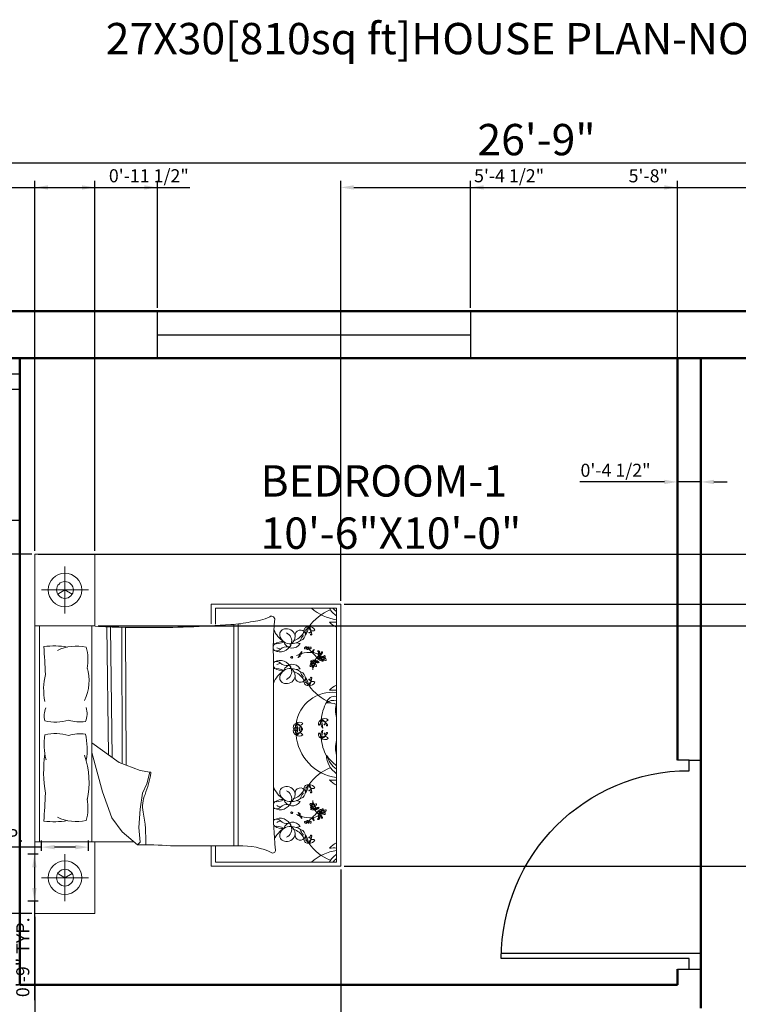
# Model space of a CAD drawing. Units: inches. Extents: x 3242 to 3618, y 1365 to 1814.
# Tile 5 of 6: x 3333 to 3471, y 1626 to 1814. Entities that reach past the tile are written whole.
import ezdxf

# ---------------------------------------------------------------- set-up
doc = ezdxf.new("R2010")
doc.units = ezdxf.units.IN
for name, color, linetype, lineweight in [('A-ANNO-DIMS', 2, 'Continuous', 18), ('A-ANNO-TEXT', 7, 'Continuous', 25), ('A-AREA-IDEN', 7, 'Continuous', 25), ('A-DOOR', 4, 'Continuous', 25), ('A-FURN', 8, 'Continuous', 18), ('A-GLAZ', 5, 'Continuous', 25), ('A-WALL', 7, 'Continuous', 50)]:
    doc.layers.add(name, color=color, linetype=linetype, lineweight=lineweight)
doc.styles.get("Standard").update_dxf_attribs({"font": 'arial.ttf'})
doc.dimstyles.new('ISO-25', dxfattribs={"dimtxt": 2.5, "dimasz": 2.5, "dimexe": 1.25, "dimexo": 0.625, "dimtad": 1, "dimdec": 0, "dimlunit": 3, "dimtxsty": 'Standard', "dimcen": 2.5, "dimadec": 0, "dimazin": 0, "dimtfac": 1, "dimtdec": 0, "dimtmove": 0, "dimatfit": 3, "dimfxl": 1, "dimarcsym": 0})

# ---------------------------------------------------------------- blocks, each defined once
blk = doc.blocks.new('*D3')
at = {"layer": 'A-ANNO-DIMS', "color": 0, "lineweight": -2, "transparency": 16777216}
for p, q in [((3271.48, 1759.28), (3271.48, 1788.3)), ((3592.48, 1759.28), (3592.48, 1788.3)), ((3273.98, 1787.05), (3589.98, 1787.05))]:
    blk.add_line(p, q, dxfattribs=at)
at = {"layer": 'A-ANNO-DIMS', "color": 0, "transparency": 16777216}
for points in [[(3273.98, 1787.47), (3273.98, 1786.64), (3271.48, 1787.05)], [(3589.98, 1787.47), (3589.98, 1786.64), (3592.48, 1787.05)]]:
    blk.add_solid(points, dxfattribs=at)
at = {"layer": 'Defpoints', "color": 0, "transparency": 16777216}
for p in [(3592.48, 1787.05), (3271.48, 1758.66), (3592.48, 1758.66)]:
    blk.add_point(p, dxfattribs=at)
at = {"layer": 'A-ANNO-DIMS', "color": 0, "transparency": 16777216, "insert": (3431.98, 1790.74), "char_height": 6, "attachment_point": 5}
blk.add_mtext('26\'-9"', dxfattribs=at)
blk = doc.blocks.new('DOOR-SWING-24IN')
for p, q in [((21.75, 28), (26.25, 28)), ((24, 28), (24, 26)), ((24, 26), (0, 26)), ((26.25, 25), (0, 25)), ((24, 2), (24, 0)), ((24, 0), (21.75, 0)), ((24, 0), (26.25, 0))]:
    blk.add_line(p, q)
blk.add_arc((24, 26), 24, 180, 270)
blk = doc.blocks.new('DOOR-SWING-36IN')
for p, q in [((33.75, 40), (38.25, 40)), ((36, 40), (36, 38)), ((36, 38), (0, 38)), ((38.25, 37), (0, 37)), ((36, 2), (36, 0)), ((36, 0), (33.75, 0)), ((36, 0), (38.25, 0))]:
    blk.add_line(p, q)
blk.add_arc((36, 38), 36, 180, 270)
blk = doc.blocks.new('WINDOW-60IN')
for p, q in [((0, 9), (60, 9)), ((0, 0), (0, 9)), ((60, 9), (60, 0)), ((0, 4.5), (60, 4.5)), ((60, 0), (0, 0))]:
    blk.add_line(p, q)
blk = doc.blocks.new('BEDSIDE-LAMP-SM')
for p, q in [((4.5, 0), (4.5, 9)), ((9, 4.5), (0, 4.5))]:
    blk.add_line(p, q)
for points in [[(4.5, 4.5), (3.11, 3.7)], [(4.5, 4.5), (5.89, 3.7)]]:
    blk.add_lwpolyline(points)
for radius in [3.21, 1.61]:
    blk.add_circle((4.5, 4.5), radius)
blk = doc.blocks.new('*D29')
at = {"layer": 'A-ANNO-DIMS', "color": 0, "lineweight": -2, "transparency": 16777216}
for p, q in [((3337.15, 1656.02), (3307.79, 1656.02)), ((3337.15, 1655.29), (3337.15, 1657.27)), ((3343.65, 1656.02), (3339.65, 1656.02)), ((3346.15, 1655.29), (3346.15, 1657.27))]:
    blk.add_line(p, q, dxfattribs=at)
at = {"layer": 'A-ANNO-DIMS', "color": 0, "transparency": 16777216}
for points in [[(3339.65, 1656.43), (3339.65, 1655.6), (3337.15, 1656.02)], [(3343.65, 1656.43), (3343.65, 1655.6), (3346.15, 1656.02)]]:
    blk.add_solid(points, dxfattribs=at)
at = {"layer": 'Defpoints', "color": 0, "transparency": 16777216}
for p in [(3337.15, 1656.02), (3337.15, 1654.67), (3346.15, 1654.67)]:
    blk.add_point(p, dxfattribs=at)
at = {"layer": 'A-ANNO-DIMS', "color": 0, "transparency": 16777216, "insert": (3321.22, 1657.92), "char_height": 2.5, "attachment_point": 5}
blk.add_mtext('LAMP 0\'-9" TYP.', dxfattribs=at)
blk = doc.blocks.new('*D30')
at = {"layer": 'A-ANNO-DIMS', "color": 0, "lineweight": -2, "transparency": 16777216}
for p, q in [((3336.53, 1654.67), (3334.55, 1654.67)), ((3335.8, 1652.17), (3335.8, 1648.17)), ((3336.53, 1645.67), (3334.55, 1645.67)), ((3335.8, 1645.67), (3335.8, 1626.68))]:
    blk.add_line(p, q, dxfattribs=at)
at = {"layer": 'A-ANNO-DIMS', "color": 0, "transparency": 16777216}
for points in [[(3335.39, 1652.17), (3336.22, 1652.17), (3335.8, 1654.67)], [(3335.39, 1648.17), (3336.22, 1648.17), (3335.8, 1645.67)]]:
    blk.add_solid(points, dxfattribs=at)
at = {"layer": 'Defpoints', "color": 0, "transparency": 16777216}
for p in [(3337.15, 1654.67), (3335.8, 1645.67), (3337.15, 1645.67)]:
    blk.add_point(p, dxfattribs=at)
at = {"layer": 'A-ANNO-DIMS', "color": 0, "transparency": 16777216, "insert": (3333.9, 1634.92), "char_height": 2.5, "attachment_point": 5, "rotation": 90}
blk.add_mtext('0\'-9" TYP.', dxfattribs=at)
blk = doc.blocks.new('*D33')
at = {"layer": 'A-ANNO-DIMS', "color": 0, "lineweight": -2, "transparency": 16777216}
for p, q in [((3271.48, 1759.28), (3271.48, 1783.61)), ((3273.98, 1782.36), (3356.86, 1782.36)), ((3359.36, 1759.28), (3359.36, 1783.61))]:
    blk.add_line(p, q, dxfattribs=at)
at = {"layer": 'A-ANNO-DIMS', "color": 0, "transparency": 16777216}
for points in [[(3273.98, 1782.77), (3273.98, 1781.94), (3271.48, 1782.36)], [(3356.86, 1782.77), (3356.86, 1781.94), (3359.36, 1782.36)]]:
    blk.add_solid(points, dxfattribs=at)
at = {"layer": 'Defpoints', "color": 0, "transparency": 16777216}
for p in [(3359.36, 1782.36), (3271.48, 1758.66), (3359.36, 1758.66)]:
    blk.add_point(p, dxfattribs=at)
at = {"layer": 'A-ANNO-DIMS', "color": 0, "transparency": 16777216, "insert": (3315.42, 1784.23), "char_height": 2.5, "attachment_point": 5}
blk.add_mtext('7\'-4"', dxfattribs=at)
blk = doc.blocks.new('*D34')
at = {"layer": 'A-ANNO-DIMS', "color": 0, "lineweight": -2, "transparency": 16777216}
for p, q in [((3419.36, 1759.28), (3419.36, 1783.61)), ((3421.86, 1782.36), (3484.93, 1782.36)), ((3487.43, 1759.28), (3487.43, 1783.61))]:
    blk.add_line(p, q, dxfattribs=at)
at = {"layer": 'A-ANNO-DIMS', "color": 0, "transparency": 16777216}
for points in [[(3421.86, 1782.77), (3421.86, 1781.94), (3419.36, 1782.36)], [(3484.93, 1782.77), (3484.93, 1781.94), (3487.43, 1782.36)]]:
    blk.add_solid(points, dxfattribs=at)
at = {"layer": 'Defpoints', "color": 0, "transparency": 16777216}
for p in [(3487.43, 1782.36), (3419.36, 1758.66), (3487.43, 1758.66)]:
    blk.add_point(p, dxfattribs=at)
at = {"layer": 'A-ANNO-DIMS', "color": 0, "transparency": 16777216, "insert": (3453.39, 1784.26), "char_height": 2.5, "attachment_point": 5}
blk.add_mtext('5\'-8"', dxfattribs=at)
blk = doc.blocks.new('*D47')
at = {"layer": 'A-ANNO-DIMS', "color": 0, "lineweight": -2, "transparency": 16777216}
for p, q in [((3458.98, 1749.03), (3458.98, 1724.71)), ((3463.48, 1749.03), (3463.48, 1724.71)), ((3456.48, 1725.96), (3440.26, 1725.96)), ((3463.48, 1725.96), (3458.98, 1725.96)), ((3465.98, 1725.96), (3468.48, 1725.96))]:
    blk.add_line(p, q, dxfattribs=at)
at = {"layer": 'A-ANNO-DIMS', "color": 0, "transparency": 16777216}
for points in [[(3456.48, 1726.37), (3456.48, 1725.54), (3458.98, 1725.96)], [(3465.98, 1726.37), (3465.98, 1725.54), (3463.48, 1725.96)]]:
    blk.add_solid(points, dxfattribs=at)
at = {"layer": 'Defpoints', "color": 0, "transparency": 16777216}
for p in [(3458.98, 1749.66), (3463.48, 1749.66), (3458.98, 1725.96)]:
    blk.add_point(p, dxfattribs=at)
at = {"layer": 'A-ANNO-DIMS', "color": 0, "transparency": 16777216, "insert": (3447.12, 1727.87), "char_height": 2.5, "attachment_point": 5}
blk.add_mtext('0\'-4 1/2"', dxfattribs=at)
blk = doc.blocks.new('*D48')
at = {"layer": 'A-ANNO-DIMS', "color": 0, "lineweight": -2, "transparency": 16777216}
for p, q in [((3394.48, 1651.75), (3394.48, 1376.71)), ((3335.91, 1642.66), (3335.91, 1376.71)), ((3338.41, 1377.96), (3391.98, 1377.96))]:
    blk.add_line(p, q, dxfattribs=at)
at = {"layer": 'A-ANNO-DIMS', "color": 0, "transparency": 16777216}
for points in [[(3338.41, 1378.37), (3338.41, 1377.54), (3335.91, 1377.96)], [(3391.98, 1378.37), (3391.98, 1377.54), (3394.48, 1377.96)]]:
    blk.add_solid(points, dxfattribs=at)
at = {"layer": 'Defpoints', "color": 0, "transparency": 16777216}
for p in [(3394.48, 1652.37), (3335.91, 1643.28), (3394.48, 1377.96)]:
    blk.add_point(p, dxfattribs=at)
at = {"layer": 'A-ANNO-DIMS', "color": 0, "transparency": 16777216, "insert": (3365.2, 1379.87), "char_height": 2.5, "attachment_point": 5}
blk.add_mtext('4\'-10 1/2"', dxfattribs=at)
blk = doc.blocks.new('*D49')
at = {"layer": 'A-ANNO-DIMS', "color": 0, "lineweight": -2, "transparency": 16777216}
for p, q in [((3395.11, 1702.58), (3617.43, 1702.58)), ((3616.18, 1700.08), (3616.18, 1654.87)), ((3395.11, 1652.37), (3617.43, 1652.37))]:
    blk.add_line(p, q, dxfattribs=at)
at = {"layer": 'A-ANNO-DIMS', "color": 0, "transparency": 16777216}
for points in [[(3615.76, 1700.08), (3616.6, 1700.08), (3616.18, 1702.58)], [(3615.76, 1654.87), (3616.6, 1654.87), (3616.18, 1652.37)]]:
    blk.add_solid(points, dxfattribs=at)
at = {"layer": 'Defpoints', "color": 0, "transparency": 16777216}
for p in [(3394.48, 1702.58), (3394.48, 1652.37), (3616.18, 1652.37)]:
    blk.add_point(p, dxfattribs=at)
at = {"layer": 'A-ANNO-DIMS', "color": 0, "transparency": 16777216, "insert": (3614.3, 1677.48), "char_height": 2.5, "attachment_point": 5, "rotation": 90}
blk.add_mtext('4\'-2"', dxfattribs=at)
blk = doc.blocks.new('*D50')
at = {"layer": 'A-ANNO-DIMS', "color": 0, "lineweight": -2, "transparency": 16777216}
for p, q in [((3348.02, 1712.15), (3617.43, 1712.15)), ((3616.18, 1709.65), (3616.18, 1700.88)), ((3348.02, 1698.38), (3617.43, 1698.38))]:
    blk.add_line(p, q, dxfattribs=at)
at = {"layer": 'A-ANNO-DIMS', "color": 0, "transparency": 16777216}
for points in [[(3615.76, 1709.65), (3616.6, 1709.65), (3616.18, 1712.15)], [(3615.76, 1700.88), (3616.6, 1700.88), (3616.18, 1698.38)]]:
    blk.add_solid(points, dxfattribs=at)
at = {"layer": 'Defpoints', "color": 0, "transparency": 16777216}
for p in [(3347.39, 1712.15), (3347.39, 1698.38), (3616.18, 1698.38)]:
    blk.add_point(p, dxfattribs=at)
at = {"layer": 'A-ANNO-DIMS', "color": 0, "transparency": 16777216, "insert": (3614.3, 1705.27), "char_height": 2.5, "attachment_point": 5, "rotation": 90}
blk.add_mtext('1\'-2"', dxfattribs=at)
blk = doc.blocks.new('*D51')
at = {"layer": 'A-ANNO-DIMS', "color": 0, "lineweight": -2, "transparency": 16777216}
for p, q in [((3335.91, 1712.78), (3335.91, 1783.61)), ((3338.41, 1782.36), (3344.89, 1782.36)), ((3347.39, 1712.78), (3347.39, 1783.61)), ((3347.39, 1782.36), (3365.56, 1782.36))]:
    blk.add_line(p, q, dxfattribs=at)
at = {"layer": 'A-ANNO-DIMS', "color": 0, "transparency": 16777216}
for points in [[(3338.41, 1782.77), (3338.41, 1781.94), (3335.91, 1782.36)], [(3344.89, 1782.77), (3344.89, 1781.94), (3347.39, 1782.36)]]:
    blk.add_solid(points, dxfattribs=at)
at = {"layer": 'Defpoints', "color": 0, "transparency": 16777216}
for p in [(3347.39, 1782.36), (3335.91, 1712.15), (3347.39, 1712.15)]:
    blk.add_point(p, dxfattribs=at)
at = {"layer": 'A-ANNO-DIMS', "color": 0, "transparency": 16777216, "insert": (3357.72, 1784.27), "char_height": 2.5, "attachment_point": 5}
blk.add_mtext('0\'-11 1/2"', dxfattribs=at)
blk = doc.blocks.new('*D52')
at = {"layer": 'A-ANNO-DIMS', "color": 0, "lineweight": -2, "transparency": 16777216}
for p, q in [((3335.29, 1712.15), (3246.53, 1712.15)), ((3247.78, 1645.78), (3247.78, 1709.65)), ((3335.29, 1643.28), (3246.53, 1643.28))]:
    blk.add_line(p, q, dxfattribs=at)
at = {"layer": 'A-ANNO-DIMS', "color": 0, "transparency": 16777216}
for points in [[(3247.36, 1709.65), (3248.2, 1709.65), (3247.78, 1712.15)], [(3247.36, 1645.78), (3248.2, 1645.78), (3247.78, 1643.28)]]:
    blk.add_solid(points, dxfattribs=at)
at = {"layer": 'Defpoints', "color": 0, "transparency": 16777216}
for p in [(3247.78, 1712.15), (3335.91, 1712.15), (3335.91, 1643.28)]:
    blk.add_point(p, dxfattribs=at)
at = {"layer": 'A-ANNO-DIMS', "color": 0, "transparency": 16777216, "insert": (3245.88, 1677.72), "char_height": 2.5, "attachment_point": 5, "rotation": 90}
blk.add_mtext('5\'-9"', dxfattribs=at)
blk = doc.blocks.new('*D58')
at = {"layer": 'A-ANNO-DIMS', "color": 0, "lineweight": -2, "transparency": 16777216}
for p, q in [((3333.61, 1749.66), (3617.43, 1749.66)), ((3616.18, 1747.16), (3616.18, 1714.65)), ((3336.54, 1712.15), (3617.43, 1712.15))]:
    blk.add_line(p, q, dxfattribs=at)
at = {"layer": 'A-ANNO-DIMS', "color": 0, "transparency": 16777216}
for points in [[(3615.76, 1747.16), (3616.6, 1747.16), (3616.18, 1749.66)], [(3615.76, 1714.65), (3616.6, 1714.65), (3616.18, 1712.15)]]:
    blk.add_solid(points, dxfattribs=at)
at = {"layer": 'Defpoints', "color": 0, "transparency": 16777216}
for p in [(3332.98, 1749.66), (3335.91, 1712.15), (3616.18, 1712.15)]:
    blk.add_point(p, dxfattribs=at)
at = {"layer": 'A-ANNO-DIMS', "color": 0, "transparency": 16777216, "insert": (3614.26, 1730.9), "char_height": 2.5, "attachment_point": 5, "rotation": 90}
blk.add_mtext('3\'-1 1/2"', dxfattribs=at)
blk = doc.blocks.new('*D60')
at = {"layer": 'A-ANNO-DIMS', "color": 0, "lineweight": -2, "transparency": 16777216}
for p, q in [((3394.48, 1703.21), (3394.48, 1783.61)), ((3396.98, 1782.36), (3456.48, 1782.36)), ((3458.98, 1673.28), (3458.98, 1783.61))]:
    blk.add_line(p, q, dxfattribs=at)
at = {"layer": 'A-ANNO-DIMS', "color": 0, "transparency": 16777216}
for points in [[(3396.98, 1782.77), (3396.98, 1781.94), (3394.48, 1782.36)], [(3456.48, 1782.77), (3456.48, 1781.94), (3458.98, 1782.36)]]:
    blk.add_solid(points, dxfattribs=at)
at = {"layer": 'Defpoints', "color": 0, "transparency": 16777216}
for p in [(3458.98, 1782.36), (3394.48, 1702.58), (3458.98, 1672.66)]:
    blk.add_point(p, dxfattribs=at)
at = {"layer": 'A-ANNO-DIMS', "color": 0, "transparency": 16777216, "insert": (3426.73, 1784.27), "char_height": 2.5, "attachment_point": 5}
blk.add_mtext('5\'-4 1/2"', dxfattribs=at)

msp = doc.modelspace()

# ---------------------------------------------------------------- linework, layer by layer
at = {"layer": 'A-FURN'}
for p, q in [((3335.91, 1643.28), (3335.91, 1712.15)), ((3369.67, 1698.76), (3369.67, 1702.58)), ((3369.67, 1702.58), (3394.48, 1702.58)), ((3370.47, 1701.78), (3370.47, 1698.75)), ((3393.69, 1701.78), (3370.47, 1701.78)), ((3393.69, 1653.17), (3393.69, 1701.78)), ((3394.48, 1702.58), (3394.48, 1652.37)), ((3336.8, 1698.38), (3336.8, 1657.06)), ((3346.8, 1657.06), (3346.8, 1698.38)), ((3349.66, 1698.19), (3350, 1673.67)), ((3350.37, 1698.17), (3350.72, 1673.16)), ((3352.53, 1698.13), (3352.64, 1671.98)), ((3353.24, 1698.13), (3353.35, 1671.71)), ((3373.97, 1698.69), (3373.97, 1656.26)), ((3374.83, 1698.76), (3374.83, 1656.26)), ((3386.7, 1695), (3385.93, 1695.15)), ((3381.59, 1691.7), (3381.59, 1663.74)), ((3386.7, 1690.18), (3385.93, 1690.03)), ((3346.8, 1675.98), (3352.05, 1672.2)), ((3348.84, 1666.62), (3346.8, 1674.13)), ((3352.05, 1672.2), (3356.09, 1670.67)), ((3356.09, 1670.67), (3357.91, 1670.39)), ((3357.91, 1670.39), (3357.35, 1668.16)), ((3357.35, 1668.16), (3356.51, 1666.34)), ((3350.66, 1661.6), (3348.84, 1666.62)), ((3356.51, 1666.34), (3356.09, 1663.27)), ((3356.09, 1663.27), (3355.81, 1659.79)), ((3386.7, 1664.77), (3385.93, 1664.92)), ((3352.61, 1658.95), (3350.66, 1661.6)), ((3355.81, 1659.79), (3356.09, 1657)), ((3386.7, 1659.96), (3385.93, 1659.8)), ((3355.54, 1656.44), (3352.61, 1658.95)), ((3335.91, 1657.06), (3354.82, 1657.06)), ((3356.09, 1657), (3355.54, 1656.44)), ((3369.67, 1652.37), (3369.67, 1656.27)), ((3370.47, 1656.27), (3370.47, 1653.17)), ((3394.48, 1652.37), (3369.67, 1652.37)), ((3370.47, 1653.17), (3393.69, 1653.17))]:
    msp.add_line(p, q, dxfattribs=at)
for points in [[(3335.91, 1698.38), (3347.39, 1698.38), (3347.39, 1712.15), (3335.91, 1712.15)], [(3347.39, 1657.06), (3347.39, 1643.28), (3335.91, 1643.28)]]:
    msp.add_lwpolyline(points, dxfattribs=at)
for points in [[(3373.43, 1698.67, 0.056112), (3377.22, 1699.17, 0.095341), (3380.87, 1700.14)], [(3337.63, 1694.42, -0.074897), (3342.13, 1694.34, 0.472817)], [(3342.38, 1680.34, -0.14099), (3337.79, 1680.2, -0.235245)], [(3342.38, 1677.39, 0.14099), (3337.79, 1677.53, 0.235245)], [(3337.63, 1661.01, 0.074897), (3342.13, 1661.09, -0.472817)], [(3361.84, 1656.29, 0.001242), (3374.91, 1656.26, -0.127202), (3381.42, 1654.88)]]:
    msp.add_lwpolyline(points, format="xyb", dxfattribs=at)
for centre in [(3391.05, 1692.16), (3389.2, 1691.02), (3389.2, 1663.94), (3391.05, 1662.79)]:
    msp.add_circle(centre, 0.175, dxfattribs=at)
for centre, radius, start, end in [((3395.79, 1693.09), 8.99, 111.4092, 145.6135), ((3394.9, 1708.48), 8.99, 228.1144, 262.255), ((3396.1, 1703.97), 4.38, 209.8884, 236.5383), ((3396.92, 1705.54), 5.46, 223.5186, 233.6964), ((3381.22, 1699.62), 0.628, 336.5219, 123.8264), ((3448.58, 1693.81), 67.02, 175.2402, 181.8035), ((3395.09, 1701.51), 3.66, 221.0454, 247.4453), ((3393.12, 1711.53), 12.44, 266.3481, 272.5919), ((3355.21, 1821.84), 123.75, 266.1, 270.9282), ((3359.71, 1859.52), 161.43, 269.1145, 274.8735), ((3386.44, 1699.71), 5.21, 203.6453, 236.3329), ((3383.94, 1696.67), 1.16, 88.9462, 185.5144), ((3384.11, 1696.19), 1.65, 7.1143, 95.0551), ((3386.76, 1696.57), 1.03, 19.1312, 189.736), ((3387.88, 1696.78), 0.634, 126.7319, 206.0245), ((3388.19, 1697.45), 0.746, 76.272, 177.0484), ((3387.05, 1698.97), 1.54, 284.7031, 328.6173), ((3389.2, 1697.02), 1.42, 125.7657, 194.5347), ((3382.22, 1699.54), 6.29, 332.8176, 347.4827), ((3388.58, 1697.2), 0.997, 20.9613, 102.2885), ((3389.12, 1698.19), 0.751, 181.7131, 301.5367), ((3386.65, 1696.67), 2.27, 2.0648, 41.1598), ((3388.02, 1697.52), 0.736, 316.2238, 62.3173), ((3388.45, 1697.09), 0.0586, 20.2667, 316.2271), ((3382.1, 1697.79), 2.85, 259.249, 301.1782), ((3383.34, 1692.72), 2.66, 85.2696, 124.215), ((3384.8, 1697.03), 2.07, 193.079, 274.7067), ((3385.22, 1695.85), 1.71, 196.8663, 330.0915), ((3383.48, 1695.55), 1.6, 338.5779, 68.4181), ((3383.74, 1696.48), 2, 305.9599, 357.6409), ((3384.75, 1698.65), 3.7, 273.4924, 303.7117), ((3384.48, 1698.62), 3.25, 288.2955, 328.7386), ((3386.45, 1696.82), 1.29, 285.6955, 4.031), ((3388.16, 1695.43), 1.37, 128.4175, 173.8338), ((3388.81, 1696.75), 0.112, 168.5166, 2.0648), ((3388.76, 1696.76), 0.0543, 52.0591, 168.5166), ((2682.19, 1656.46), 656.53, 2.85022, 3.31479), ((3343.93, 1685.65), 8.88, 78.2417, 114.8684), ((3336.82, 1691.97), 9.23, 348.9631, 14.8961), ((3382.36, 1694.26), 0.829, 127.675, 162.5814), ((3382.36, 1694.26), 0.829, 196.6343, 225.5483), ((3382.85, 1695.58), 2.19, 240.8249, 340.7178), ((3382.19, 1694.61), 1.03, 246.1646, 318.4347), ((3383.24, 1695.92), 1.98, 240.0851, 262.564), ((3384.02, 1692.99), 1.41, 74.8529, 138.4347), ((3384.5, 1694.77), 0.427, 254.8529, 12.6959), ((3383.34, 1692.72), 2.66, 53.6555, 57.2989), ((3387.2, 1693.15), 0.362, 115.5379, 168.6744), ((3385.97, 1693.67), 1.09, 329.344, 349.7412), ((3385.1, 1693.42), 1.94, 352.8698, 1.6736), ((3387.68, 1694.12), 0.136, 125.0752, 284.7644), ((3387.89, 1694.18), 0.293, 127.3642, 168.4363), ((3387.66, 1694.41), 0.422, 277.4968, 341.2737), ((3387.99, 1694.21), 0.168, 88.1325, 178.8919), ((3388.33, 1694.04), 0.363, 136.3462, 189.6513), ((3388.12, 1694), 0.151, 189.6513, 312.3208), ((3388.16, 1694.42), 0.175, 183.2768, 356.7232), ((3388.71, 1694.1), 0.574, 164.2829, 186.9148), ((3388.03, 1694.1), 0.287, 312.3208, 40.2111), ((3388.64, 1694.42), 0.408, 201.6382, 274.947), ((3388.1, 1693.87), 0.533, 42.3896, 66.5724), ((3393.47, 1698.08), 6.54, 217.9541, 226.8459), ((3388.48, 1694.18), 0.29, 10.9597, 52.2379), ((3388.66, 1694.15), 0.135, 274.947, 37.5263), ((3389.11, 1693.39), 0.14, 112.5583, 214.2343), ((3389.02, 1693.64), 0.331, 265.7131, 351.6568), ((3388.73, 1693.82), 0.577, 297.3659, 329.344), ((3388.29, 1694.32), 1.11, 313.6929, 321.7899), ((3389.52, 1693.56), 0.362, 115.5379, 168.6744), ((3388.29, 1694.08), 1.09, 329.344, 349.7412), ((3387.42, 1693.83), 1.94, 352.8698, 1.6736), ((3390.15, 1693.44), 0.196, 33.0979, 123.1364), ((3385.84, 1690.68), 5.12, 31.1156, 34.8118), ((3389.87, 1693.11), 0.53, 2.3172, 70.5201), ((3390.05, 1693.22), 0.203, 315.7354, 31.1156), ((3390.07, 1693.16), 0.457, 352.6008, 57.1845), ((3390.37, 1693.43), 0.53, 291.7087, 3.0299), ((3386.59, 1696.22), 5.12, 323.6254, 327.3216), ((3390.79, 1693.3), 0.196, 325.6077, 55.6462), ((3382.36, 1690.92), 0.829, 134.4517, 156.7144), ((3382.85, 1689.6), 2.19, 19.2822, 119.1751), ((3382.19, 1690.57), 1.03, 41.5653, 113.8354), ((3385.07, 1692.41), 0.216, 169.5864, 349.5616), ((3385.15, 1692.39), 0.133, 349.5616, 167.2949), ((3388.62, 1687.62), 5.7, 110.1059, 116.9968), ((3386.7, 1692.32), 0.362, 129.5056, 182.6421), ((3385.66, 1693.16), 1.09, 308.4388, 328.836), ((3385.47, 1694.04), 1.94, 296.5064, 305.3102), ((3385.46, 1693.04), 1.11, 336.3901, 344.4871), ((3386.66, 1692.76), 0.14, 83.9457, 185.6216), ((3386.1, 1692.89), 0.577, 328.836, 0.8141), ((3386.4, 1692.72), 0.331, 306.5232, 32.4668), ((3386.79, 1692.98), 0.14, 112.5583, 214.2343), ((3386.7, 1693.23), 0.331, 265.7131, 351.6568), ((3386.41, 1693.41), 0.577, 297.3659, 329.344), ((3385.98, 1693.91), 1.11, 313.6929, 321.7899), ((3388.62, 1687.62), 5.7, 86.1723, 106.4158), ((3388.94, 1692.36), 0.799, 253.6301, 325.4631), ((3389.16, 1691.25), 0.566, 82.0748, 142.6895), ((3389.1, 1692.03), 0.581, 228.342, 274.9894), ((3388.96, 1691.21), 0.239, 358.5719, 143.8954), ((3388.76, 1690.46), 2.86, 60.7959, 85.244), ((3382.67, 1686.34), 9.41, 37.8256, 47.7588), ((3389.12, 1691.93), 0.486, 273.8774, 357.1501), ((3389.73, 1691.06), 0.553, 121.9501, 165.2442), ((3389.31, 1692.28), 0.471, 262.0748, 308.2393), ((3389.33, 1691.37), 0.346, 278.5614, 22.5914), ((3392.56, 1690.17), 3.43, 156.1523, 156.9499), ((3389.53, 1691.39), 0.174, 44.3732, 121.9501), ((3390.07, 1691.79), 0.486, 181.4625, 249.4747), ((3392.56, 1690.17), 3.43, 130.182, 149.456), ((3389.98, 1692.18), 0.471, 215.1128, 261.2773), ((3390.36, 1692.15), 0.799, 197.889, 269.722), ((3389.83, 1691.15), 0.566, 20.6625, 81.2773), ((3390.67, 1692.12), 0.566, 139.3812, 199.9959), ((3389.61, 1692.53), 0.799, 310.9365, 22.7695), ((3389.98, 1692.49), 0.581, 285.6484, 332.2957), ((3390.31, 1692.97), 0.153, 135.7354, 318.1297), ((3389.88, 1692.79), 0.471, 319.3812, 5.5456), ((3390.42, 1692.98), 0.153, 68.2452, 250.6395), ((3391.7, 1690.1), 3.05, 111.7087, 116.2181), ((3388.76, 1690.46), 2.86, 47.5083, 55.9967), ((3390.5, 1693.27), 0.457, 252.8042, 349.6943), ((3390.07, 1692.45), 0.486, 331.1838, 51.6792), ((3390.57, 1691.87), 0.136, 125.0752, 284.7644), ((3390.55, 1693.31), 0.203, 248.2452, 323.6254), ((3390.78, 1691.92), 0.293, 93.635, 168.4363), ((3390.74, 1692.39), 0.172, 138.2946, 276.2474), ((3390.55, 1692.16), 0.422, 277.4968, 341.2737), ((3390.8, 1692.36), 0.239, 358.5719, 143.8954), ((3390.88, 1691.96), 0.168, 88.1325, 178.8919), ((3390.94, 1692.55), 0.241, 208.8493, 269.9355), ((3390.74, 1692.49), 0.276, 274.2123, 318.1587), ((3391.22, 1691.78), 0.363, 136.3462, 189.6513), ((3391.01, 1691.75), 0.151, 189.6513, 312.3208), ((3391.6, 1691.85), 0.574, 164.2829, 186.9148), ((3391.58, 1692.21), 0.553, 121.9501, 165.2442), ((3390.92, 1691.85), 0.287, 312.3208, 40.2111), ((3391.53, 1692.17), 0.408, 201.6382, 274.947), ((3391.2, 1692.42), 0.116, 262.868, 7.094), ((3390.99, 1691.61), 0.533, 42.3896, 66.5724), ((3391.18, 1692.52), 0.346, 278.5614, 22.5914), ((3391.37, 1691.93), 0.29, 10.9597, 118.7804), ((3391.38, 1692.53), 0.174, 44.3732, 121.9501), ((3391.55, 1691.9), 0.135, 274.947, 37.5263), ((3337.5, 1687.98), 8.77, 333.8761, 16.1746), ((3382.36, 1690.92), 0.829, 203.2856, 232.325), ((3382.1, 1687.39), 2.85, 58.8218, 100.2867), ((3386.44, 1685.47), 5.21, 123.6671, 158.5059), ((3383.34, 1692.46), 2.66, 235.785, 274.7304), ((3383.24, 1689.26), 1.98, 97.436, 119.9149), ((3384.8, 1688.15), 2.07, 85.2933, 166.921), ((3384.02, 1692.19), 1.41, 221.5653, 285.1471), ((3385.22, 1689.33), 1.71, 29.9085, 163.1337), ((3383.48, 1689.63), 1.6, 291.5819, 21.4221), ((3384.5, 1690.41), 0.427, 347.3041, 105.1471), ((3383.34, 1692.46), 2.66, 302.7011, 306.3445), ((3383.74, 1688.7), 2, 2.3591, 54.0401), ((3384.75, 1686.53), 3.7, 56.2883, 86.5076), ((3384.48, 1686.56), 3.25, 31.2614, 71.7045), ((3388.16, 1689.75), 1.37, 186.1662, 231.5825), ((3386.45, 1688.36), 1.29, 355.969, 74.3045), ((3388.72, 1690.72), 0.136, 125.0752, 284.7644), ((3388.93, 1690.78), 0.293, 93.635, 168.4363), ((3388.89, 1691.24), 0.172, 138.2946, 276.2474), ((3388.7, 1691.01), 0.422, 277.4968, 341.2737), ((3389.03, 1690.81), 0.168, 88.1325, 178.8919), ((3389.09, 1691.4), 0.241, 208.8493, 269.9355), ((3388.89, 1691.34), 0.276, 274.2123, 318.1587), ((3389.37, 1690.64), 0.363, 136.3462, 189.6513), ((3389.16, 1690.6), 0.151, 189.6513, 312.3208), ((3392.56, 1690.17), 3.43, 175.2415, 182.8929), ((3389.75, 1690.7), 0.574, 164.2829, 186.9148), ((3389.07, 1690.7), 0.287, 312.3208, 40.2111), ((3389.68, 1691.02), 0.408, 201.6382, 274.947), ((3389.35, 1691.28), 0.116, 262.868, 7.094), ((3389.14, 1690.47), 0.533, 42.3896, 66.5724), ((3389.52, 1690.78), 0.29, 10.9597, 118.7804), ((3389.7, 1690.75), 0.135, 274.947, 37.5263), ((3390.11, 1691.88), 0.581, 248.3627, 295.0101), ((3349.68, 1686.25), 12.11, 166.3427, 191.1841), ((3383.94, 1688.51), 1.16, 174.4856, 271.0538), ((3384.11, 1688.99), 1.65, 264.9449, 352.8857), ((3386.76, 1688.61), 1.03, 170.264, 340.8688), ((3387.88, 1688.4), 0.634, 153.9755, 233.2681), ((3388.19, 1687.73), 0.746, 182.9516, 283.728), ((3387.05, 1686.21), 1.54, 31.3827, 75.2969), ((3389.2, 1688.16), 1.42, 165.4653, 234.2343), ((3382.22, 1685.64), 6.29, 12.5173, 27.1824), ((3386.65, 1688.51), 2.27, 318.8402, 357.9352), ((3388.02, 1687.66), 0.736, 297.6827, 43.7762), ((3389.12, 1686.99), 0.751, 58.4633, 178.2869), ((3388.48, 1688.1), 0.0973, 43.7762, 339.7183), ((3388.81, 1688.43), 0.112, 357.9352, 191.4834), ((3388.76, 1688.42), 0.0543, 191.4834, 307.9409), ((3388.58, 1687.98), 0.997, 257.7115, 339.0387), ((3395.79, 1692.09), 8.99, 214.3865, 248.5908), ((3395.09, 1683.67), 3.66, 112.5547, 138.9546), ((3393.12, 1673.65), 12.44, 87.4081, 93.6519), ((3392.82, 1678.71), 6.96, 82.8636, 171.8197), ((3393.31, 1683.3), 1.61, 76.3898, 169.0739), ((3393.08, 1682.09), 2.04, 72.8609, 131.9049), ((3341.06, 1681.14), 3.41, 153.3437, 196.1026), ((3342.25, 1681.6), 3.65, 335.0183, 18.5407), ((3399.72, 1679.68), 8.99, 152.5854, 175.5377), ((3392.19, 1679.61), 4.03, 68.117, 96.6195), ((3398.42, 1682.2), 4.95, 162.9798, 196.4569), ((3344.68, 1688.45), 8.44, 254.1707, 275.9871), ((3390.96, 1679.67), 0.746, 106.1963, 206.9726), ((3389.21, 1680.42), 1.54, 314.6273, 358.5415), ((3392.04, 1679.8), 1.42, 155.6899, 224.4589), ((3391.42, 1679.65), 0.997, 50.8855, 132.2127), ((3391.39, 1680.78), 0.751, 211.6373, 331.4609), ((3390.78, 1679.65), 0.736, 346.148, 92.2415), ((3390.01, 1678.23), 2.27, 31.989, 71.0841), ((3384.75, 1678.5), 6.29, 2.7418, 17.407), ((3400.96, 1680.24), 7.31, 174.3643, 175.6213), ((3405.97, 1676.39), 13.07, 160.0972, 160.2783), ((3386.14, 1678.98), 0.746, 106.1963, 206.9726), ((3386.14, 1678.27), 0.746, 153.0274, 253.8037), ((3384.4, 1679.74), 1.54, 314.6273, 358.5415), ((3384.4, 1677.51), 1.54, 1.4585, 45.3727), ((3387.23, 1679.11), 1.42, 155.6899, 224.4589), ((3387.23, 1678.14), 1.42, 135.5411, 204.3101), ((3386.6, 1678.96), 0.997, 50.8855, 132.2127), ((3386.57, 1680.09), 0.751, 211.6373, 331.4609), ((3385.96, 1678.96), 0.736, 346.148, 92.2415), ((3385.19, 1677.54), 2.27, 31.989, 71.0841), ((3379.93, 1677.81), 6.29, 2.7418, 17.407), ((3379.93, 1679.43), 6.29, 342.593, 357.2582), ((3385.19, 1679.7), 2.27, 288.9159, 328.011), ((3385.96, 1678.29), 0.736, 267.7585, 13.852), ((3386.54, 1678.8), 0.0586, 50.1909, 346.0209), ((3386.58, 1678.44), 0.0973, 13.852, 309.9245), ((3387.03, 1678.69), 0.112, 198.4408, 31.989), ((3386.97, 1678.67), 0.0543, 81.9833, 198.4408), ((3387.03, 1678.56), 0.112, 328.011, 161.5592), ((3386.97, 1678.58), 0.0543, 161.5592, 278.0167), ((3392.04, 1677.45), 1.42, 135.5411, 204.3101), ((3384.75, 1678.75), 6.29, 342.593, 357.2582), ((3391.36, 1679.49), 0.0586, 50.1909, 346.0209), ((3391.85, 1679.38), 0.112, 198.4408, 31.989), ((3391.79, 1679.36), 0.0543, 81.9833, 198.4408), ((3349.93, 1675.72), 12.27, 171.5249, 193.96), ((3344.68, 1669.28), 8.44, 84.0129, 105.8293), ((3333.76, 1674.81), 12.15, 349.8617, 13.6238), ((3386.57, 1677.16), 0.751, 28.5391, 148.3627), ((3386.6, 1678.29), 0.997, 227.7873, 309.1145), ((3394.9, 1678.25), 8.99, 184.4623, 262.255), ((3390.96, 1677.58), 0.746, 153.0274, 253.8037), ((3389.21, 1676.82), 1.54, 1.4585, 45.3727), ((3390.01, 1679.02), 2.27, 288.9159, 328.011), ((3390.78, 1677.6), 0.736, 267.7585, 13.852), ((3391.39, 1676.47), 0.751, 28.5391, 148.3627), ((3391.42, 1677.6), 0.997, 227.7873, 309.1145), ((3399.72, 1677.56), 8.99, 184.4623, 207.4146), ((3391.4, 1677.75), 0.0973, 13.852, 309.9245), ((3391.85, 1677.87), 0.112, 328.011, 161.5592), ((3391.79, 1677.89), 0.0543, 161.5592, 278.0167), ((3398.42, 1675.05), 4.95, 163.5431, 197.0202), ((3400.96, 1677.01), 7.31, 184.3787, 185.6357), ((3405.97, 1680.86), 13.07, 199.7217, 199.9028), ((3362.55, 1670.45), 24.98, 172.2196, 189.497), ((3330.26, 1668.33), 16.01, 348.0397, 19.2615), ((3396.1, 1673.74), 4.38, 181.272, 236.5383), ((3398.46, 1678.19), 8.12, 214.0123, 234.053), ((3396.92, 1675.32), 5.46, 197.8504, 233.6964), ((3395.79, 1662.87), 8.99, 111.4092, 145.6135), ((3331.88, 1675.17), 26.71, 340.1194, 349.3383), ((3357.96, 1670.23), 0.166, 358.8623, 109.7536), ((3393.12, 1681.3), 12.44, 266.3481, 272.5919), ((3395.09, 1671.29), 3.66, 221.0454, 247.4453), ((3386.44, 1669.48), 5.21, 201.4941, 236.3329), ((3383.94, 1666.44), 1.16, 88.9462, 185.5144), ((3384.11, 1665.97), 1.65, 7.1143, 95.0551), ((3386.76, 1666.34), 1.03, 19.1312, 189.736), ((3387.88, 1666.56), 0.634, 126.7319, 206.0245), ((3388.19, 1667.22), 0.746, 76.272, 177.0484), ((3387.05, 1668.74), 1.54, 284.7031, 328.6173), ((3389.2, 1666.79), 1.42, 125.7657, 194.5347), ((3382.22, 1669.31), 6.29, 332.8176, 347.4827), ((3388.58, 1666.97), 0.997, 20.9613, 102.2885), ((3388.02, 1667.29), 0.736, 316.2238, 62.3173), ((3386.65, 1666.45), 2.27, 2.0648, 41.1598), ((3389.12, 1667.97), 0.751, 181.7131, 301.5367), ((2682.19, 1698.97), 656.53, 356.68521, 357.14978), ((3336.82, 1663.47), 9.23, 345.1039, 11.0369), ((3362.13, 1663.83), 5.61, 156.2616, 191.3392), ((3382.1, 1667.57), 2.85, 259.7133, 301.1782), ((3383.34, 1662.49), 2.66, 85.2696, 124.215), ((3384.8, 1666.8), 2.07, 193.079, 274.7067), ((3385.22, 1665.62), 1.71, 196.8663, 330.0915), ((3383.48, 1665.32), 1.6, 338.5779, 68.4181), ((3383.74, 1666.25), 2, 305.9599, 357.6409), ((3384.75, 1668.42), 3.7, 273.4924, 303.7117), ((3384.48, 1668.39), 3.25, 288.2955, 328.7386), ((3386.45, 1666.59), 1.29, 285.6955, 4.031), ((3388.16, 1665.2), 1.37, 128.4175, 173.8338), ((3388.45, 1666.86), 0.0586, 20.2667, 316.2271), ((3388.81, 1666.53), 0.112, 168.5166, 2.0648), ((3388.76, 1666.54), 0.0543, 52.0591, 168.5166), ((3382.36, 1664.03), 0.829, 127.675, 156.7144), ((3453.29, 1662.91), 71.7, 179.3433, 185.6887), ((3382.36, 1664.03), 0.829, 203.229, 225.5483), ((3382.85, 1665.36), 2.19, 240.8249, 340.7178), ((3382.19, 1664.38), 1.03, 246.1646, 318.4347), ((3383.24, 1665.69), 1.98, 240.0851, 262.564), ((3384.02, 1662.76), 1.41, 74.8529, 138.4347), ((3384.5, 1664.54), 0.427, 254.8529, 12.6959), ((3383.34, 1662.49), 2.66, 53.6555, 57.2989), ((3388.72, 1664.23), 0.136, 75.2356, 234.9248), ((3388.93, 1664.18), 0.293, 191.5637, 266.365), ((3389.1, 1662.93), 0.581, 85.0106, 131.658), ((3388.94, 1662.59), 0.799, 34.5369, 106.3699), ((3389.16, 1663.7), 0.566, 217.3105, 277.9252), ((3388.89, 1663.71), 0.172, 83.7526, 221.7054), ((3388.7, 1663.94), 0.422, 18.7263, 82.5032), ((3388.96, 1663.74), 0.239, 216.1046, 1.4281), ((3389.03, 1664.14), 0.168, 181.1081, 271.8675), ((3389.09, 1663.55), 0.241, 90.0645, 151.1507), ((3388.89, 1663.61), 0.276, 41.8413, 85.7877), ((3389.16, 1664.35), 0.151, 47.6792, 170.3487), ((3389.37, 1664.32), 0.363, 170.3487, 223.6538), ((3392.56, 1664.79), 3.43, 177.1071, 184.7585), ((3389.12, 1663.02), 0.486, 2.8499, 86.1226), ((3389.75, 1664.25), 0.574, 173.0852, 195.7171), ((3389.73, 1663.89), 0.553, 194.7558, 238.0499), ((3389.07, 1664.25), 0.287, 319.7889, 47.6792), ((3389.68, 1663.93), 0.408, 85.053, 158.3618), ((3389.35, 1663.68), 0.116, 352.906, 97.132), ((3389.14, 1664.49), 0.533, 293.4276, 317.6104), ((3389.52, 1664.17), 0.29, 241.2196, 349.0403), ((3389.33, 1663.58), 0.346, 337.4086, 81.4386), ((3392.56, 1664.79), 3.43, 203.0501, 203.8477), ((3389.53, 1663.57), 0.174, 238.0499, 315.6268), ((3390.07, 1663.16), 0.486, 110.5253, 178.5375), ((3390.36, 1662.8), 0.799, 90.278, 162.111), ((3389.98, 1662.77), 0.471, 98.7227, 144.8872), ((3389.7, 1664.2), 0.135, 322.4737, 85.053), ((3390.11, 1663.07), 0.581, 64.9899, 111.6373), ((3389.83, 1663.8), 0.566, 278.7227, 339.3375), ((3390.57, 1663.08), 0.136, 75.2356, 234.9248), ((3390.55, 1662.8), 0.422, 18.7263, 82.5032), ((3391.01, 1663.21), 0.151, 47.6792, 170.3487), ((3391.22, 1663.17), 0.363, 170.3487, 223.6538), ((3391.6, 1663.1), 0.574, 173.0852, 195.7171), ((3390.92, 1663.11), 0.287, 319.7889, 47.6792), ((3391.53, 1662.78), 0.408, 85.053, 158.3618), ((3391.55, 1663.05), 0.135, 322.4737, 85.053), ((3343.93, 1669.79), 8.88, 245.1316, 281.7583), ((3331.15, 1657.62), 25.99, 357.4519, 11.3392), ((3382.36, 1660.69), 0.829, 134.4517, 153.558), ((3382.85, 1659.37), 2.19, 19.2822, 119.1751), ((3382.19, 1660.34), 1.03, 41.5653, 113.8354), ((3385.07, 1662.55), 0.216, 10.4384, 190.4136), ((3385.15, 1662.56), 0.133, 192.7051, 10.4384), ((3388.62, 1667.33), 5.7, 243.0032, 249.8941), ((3385.66, 1661.8), 1.09, 31.164, 51.5612), ((3386.7, 1662.63), 0.362, 177.3579, 230.4944), ((3385.47, 1660.91), 1.94, 54.6898, 63.4936), ((3385.46, 1661.91), 1.11, 15.5129, 23.6099), ((3386.66, 1662.19), 0.14, 174.3784, 276.0543), ((3386.4, 1662.23), 0.331, 327.5332, 53.4768), ((3386.1, 1662.06), 0.577, 359.1859, 31.164), ((3386.79, 1661.97), 0.14, 145.7657, 247.4417), ((3386.7, 1661.72), 0.331, 8.3432, 94.2869), ((3386.41, 1661.54), 0.577, 30.656, 62.6341), ((3385.98, 1661.04), 1.11, 38.2101, 46.3071), ((3387.2, 1661.8), 0.362, 191.3256, 244.4621), ((3385.97, 1661.28), 1.09, 10.2588, 30.656), ((3388.62, 1667.33), 5.7, 253.5842, 273.8277), ((3385.1, 1661.53), 1.94, 358.3264, 7.1302), ((3393.47, 1656.87), 6.54, 133.1541, 142.0459), ((3389.11, 1661.56), 0.14, 145.7657, 247.4417), ((3382.67, 1668.61), 9.41, 312.2412, 322.1744), ((3388.76, 1664.49), 2.86, 274.756, 299.2041), ((3389.02, 1661.31), 0.331, 8.3432, 94.2869), ((3388.73, 1661.13), 0.577, 30.656, 62.6341), ((3388.29, 1660.63), 1.11, 38.2101, 46.3071), ((3389.52, 1661.39), 0.362, 191.3256, 244.4621), ((3388.29, 1660.87), 1.09, 10.2588, 30.656), ((3389.31, 1662.68), 0.471, 51.7607, 97.9252), ((3387.42, 1661.12), 1.94, 358.3264, 7.1302), ((3392.56, 1664.79), 3.43, 210.544, 229.818), ((3389.87, 1661.85), 0.53, 289.4799, 357.6828), ((3385.84, 1664.27), 5.12, 325.1882, 328.8844), ((3390.15, 1661.51), 0.196, 236.8636, 326.9021), ((3390.67, 1662.83), 0.566, 160.0041, 220.6188), ((3389.61, 1662.42), 0.799, 337.2305, 49.0635), ((3389.98, 1662.47), 0.581, 27.7043, 74.3516), ((3390.31, 1661.98), 0.153, 41.8703, 224.2646), ((3390.05, 1661.73), 0.203, 328.8844, 44.2646), ((3389.88, 1662.16), 0.471, 354.4544, 40.6188), ((3390.42, 1661.98), 0.153, 109.3605, 291.7548), ((3390.07, 1661.79), 0.457, 302.8155, 7.3992), ((3391.7, 1664.85), 3.05, 243.7819, 248.2913), ((3388.76, 1664.49), 2.86, 304.0033, 312.4917), ((3390.07, 1662.5), 0.486, 308.3208, 28.8162), ((3390.5, 1661.69), 0.457, 10.3057, 107.1958), ((3390.55, 1661.65), 0.203, 36.3746, 111.7548), ((3390.78, 1663.03), 0.293, 191.5637, 266.365), ((3390.74, 1662.57), 0.172, 83.7526, 221.7054), ((3390.37, 1661.52), 0.53, 356.9701, 68.2913), ((3390.8, 1662.59), 0.239, 216.1046, 1.4281), ((3390.88, 1662.99), 0.168, 181.1081, 271.8675), ((3386.59, 1658.73), 5.12, 32.6784, 36.3746), ((3390.94, 1662.41), 0.241, 90.0645, 151.1507), ((3390.74, 1662.46), 0.276, 41.8413, 85.7877), ((3390.79, 1661.66), 0.196, 304.3538, 34.3923), ((3391.58, 1662.74), 0.553, 194.7558, 238.0499), ((3391.2, 1662.53), 0.116, 352.906, 97.132), ((3390.99, 1663.34), 0.533, 293.4276, 317.6104), ((3391.37, 1663.03), 0.29, 241.2196, 349.0403), ((3391.18, 1662.43), 0.346, 337.4086, 81.4386), ((3391.38, 1662.42), 0.174, 238.0499, 315.6268), ((3382.36, 1660.69), 0.829, 210.0293, 232.325), ((3382.1, 1657.16), 2.85, 58.8218, 99.1554), ((3386.44, 1655.25), 5.21, 123.6671, 153.2997), ((3383.34, 1662.23), 2.66, 235.785, 274.7304), ((3383.24, 1659.04), 1.98, 97.436, 119.9149), ((3384.8, 1657.93), 2.07, 85.2933, 166.921), ((3384.02, 1661.96), 1.41, 221.5653, 285.1471), ((3385.22, 1659.1), 1.71, 29.9085, 163.1337), ((3383.48, 1659.41), 1.6, 291.5819, 21.4221), ((3384.5, 1660.19), 0.427, 347.3041, 105.1471), ((3383.34, 1662.23), 2.66, 302.7011, 306.3445), ((3383.74, 1658.47), 2, 2.3591, 54.0401), ((3384.75, 1656.3), 3.7, 56.2883, 86.5076), ((3384.48, 1656.33), 3.25, 31.2614, 71.7045), ((3387.68, 1660.83), 0.136, 75.2356, 234.9248), ((3387.89, 1660.78), 0.293, 191.5637, 232.6358), ((3387.66, 1660.54), 0.422, 18.7263, 82.5032), ((3387.99, 1660.74), 0.168, 181.1081, 271.8675), ((3388.12, 1660.95), 0.151, 47.6792, 170.3487), ((3388.33, 1660.92), 0.363, 170.3487, 223.6538), ((3388.16, 1660.53), 0.175, 3.2768, 176.7232), ((3388.71, 1660.85), 0.574, 173.0852, 195.7171), ((3388.03, 1660.85), 0.287, 319.7889, 47.6792), ((3388.64, 1660.53), 0.408, 85.053, 158.3618), ((3388.1, 1661.09), 0.533, 293.4276, 317.6104), ((3388.48, 1660.77), 0.29, 307.7621, 349.0403), ((3388.66, 1660.8), 0.135, 322.4737, 85.053), ((3383.94, 1658.28), 1.16, 174.4856, 271.0538), ((3384.11, 1658.76), 1.65, 264.9449, 352.8857), ((3386.76, 1658.38), 1.03, 170.264, 340.8688), ((3386.45, 1658.13), 1.29, 355.969, 74.3045), ((3388.16, 1659.52), 1.37, 186.1662, 231.5825), ((3387.88, 1658.17), 0.634, 153.9755, 233.2681), ((3389.2, 1657.93), 1.42, 165.4653, 234.2343), ((3382.22, 1655.42), 6.29, 12.5173, 27.1824), ((3386.65, 1658.28), 2.27, 318.8402, 357.9352), ((3388.02, 1657.43), 0.736, 297.6827, 43.7762), ((3389.12, 1656.76), 0.751, 58.4633, 178.2869), ((3388.48, 1657.87), 0.0973, 43.7762, 339.7183), ((3388.81, 1658.2), 0.112, 357.9352, 191.4834), ((3388.76, 1658.19), 0.0543, 191.4834, 307.9409), ((3357.25, 1593.29), 63.17, 85.8294, 91.553), ((3381.38, 1655.51), 0.635, 273.98, 27.3412), ((3387.05, 1655.98), 1.54, 31.3827, 75.2969), ((3388.19, 1657.51), 0.746, 182.9516, 283.728), ((3388.58, 1657.76), 0.997, 257.7115, 339.0387), ((3395.79, 1661.86), 8.99, 214.3865, 248.5908), ((3395.09, 1653.44), 3.66, 112.5547, 138.9546), ((3393.12, 1643.42), 12.44, 87.4081, 93.6519), ((3394.9, 1646.47), 8.99, 97.745, 131.8856), ((3396.1, 1650.99), 4.38, 123.4617, 150.1116), ((3396.92, 1649.41), 5.46, 126.3036, 136.4814)]:
    msp.add_arc(centre, radius, start, end, dxfattribs=at)
at = {"layer": 'A-WALL'}
for p, q in [((3271.48, 1758.66), (3592.48, 1758.66)), ((3280.48, 1749.66), (3583.48, 1749.66)), ((3332.98, 1749.66), (3332.98, 1629.66)), ((3458.98, 1749.66), (3458.98, 1672.66)), ((3463.48, 1749.66), (3463.48, 1625.16)), ((3458.98, 1632.66), (3458.98, 1629.66)), ((3332.98, 1629.66), (3458.98, 1629.66))]:
    msp.add_line(p, q, dxfattribs=at)

# ---------------------------------------------------------------- block references
at = {"layer": 'A-DOOR'}
msp.add_blockref('DOOR-SWING-24IN', (3306.73, 1718.65), dxfattribs=at)
at = {"layer": 'A-DOOR', "extrusion": (0, 0, -1), "zscale": -1, "rotation": 180}
msp.add_blockref('DOOR-SWING-36IN', (-3425.23, 1672.66), dxfattribs=at)
at = {"layer": 'A-FURN'}
msp.add_blockref('BEDSIDE-LAMP-SM', (3337.15, 1700.77), dxfattribs=at)
at = {"layer": 'A-FURN', "rotation": 180}
msp.add_blockref('BEDSIDE-LAMP-SM', (3346.15, 1654.67), dxfattribs=at)
at = {"layer": 'A-GLAZ'}
msp.add_blockref('WINDOW-60IN', (3359.36, 1749.65), dxfattribs=at)

# ---------------------------------------------------------------- texts
at = {"layer": 'A-ANNO-TEXT', "insert": (3349.47, 1813.86), "char_height": 6, "attachment_point": 1}
msp.add_mtext('27X30[810sq ft]HOUSE PLAN-NORTH FACE-FP1060', dxfattribs=at)
at = {"layer": 'A-AREA-IDEN', "insert": (3379.12, 1729.15), "char_height": 6, "attachment_point": 1}
msp.add_mtext('BEDROOM-1\\P10\'-6"X10\'-0"', dxfattribs=at)

# ---------------------------------------------------------------- dimensions: what is measured, and where the dimension line sits
at = {"layer": 'A-ANNO-DIMS'}
for base, p1, p2, override, picture, middle in [((3592.48, 1787.05), (3271.48, 1758.66), (3592.48, 1758.66), {"dimtxt": 6, "dimclrd": 0, "dimclre": 0, "dimclrt": 0}, '*D3', (3431.98, 1790.74)), ((3347.39, 1782.36), (3335.91, 1712.15), (3347.39, 1712.15), {"dimdec": 1, "dimlfac": 1, "dimrnd": 0, "dimzin": 1, "dimdsep": 46, "dimlunit": 4, "dimfrac": 2}, '*D51', (3357.72, 1784.27)), ((3458.98, 1782.36), (3394.48, 1702.58), (3458.98, 1672.66), {"dimdec": 1, "dimlfac": 1, "dimrnd": 0, "dimzin": 1, "dimdsep": 46, "dimlunit": 4, "dimfrac": 2}, '*D60', (3426.73, 1784.27)), ((3359.36, 1782.36), (3271.48, 1758.66), (3359.36, 1758.66), {"dimdec": 1, "dimlfac": 1, "dimrnd": 0, "dimzin": 1, "dimdsep": 46, "dimlunit": 4, "dimfrac": 2}, '*D33', (3315.42, 1784.23)), ((3487.43, 1782.36), (3419.36, 1758.66), (3487.43, 1758.66), {"dimdec": 1, "dimlfac": 1, "dimrnd": 0, "dimzin": 1, "dimdsep": 46, "dimlunit": 4, "dimfrac": 2}, '*D34', (3453.39, 1784.26)), ((3394.48, 1377.96), (3335.91, 1643.28), (3394.48, 1652.37), {"dimdec": 1, "dimlfac": 1, "dimrnd": 0, "dimzin": 1, "dimdsep": 46, "dimlunit": 4, "dimfrac": 2}, '*D48', (3365.2, 1379.87))]:
    dim = msp.add_linear_dim(base=base, p1=p1, p2=p2, dimstyle='ISO-25', override=override, dxfattribs=at)
    dim.commit()
    dim.dimension.update_dxf_attribs({"geometry": picture, "text_midpoint": middle})
for base, p1, p2, angle, picture, middle in [((3616.18, 1712.15), (3332.98, 1749.66), (3335.91, 1712.15), 90, '*D58', (3614.26, 1730.9)), ((3458.98, 1725.96), (3463.48, 1749.66), (3458.98, 1749.66), 180, '*D47', (3447.12, 1727.87)), ((3247.78, 1712.15), (3335.91, 1643.28), (3335.91, 1712.15), 90, '*D52', (3245.88, 1677.72)), ((3616.18, 1698.38), (3347.39, 1712.15), (3347.39, 1698.38), 90, '*D50', (3614.3, 1705.27)), ((3616.18, 1652.37), (3394.48, 1702.58), (3394.48, 1652.37), 90, '*D49', (3614.3, 1677.48))]:
    dim = msp.add_linear_dim(base=base, p1=p1, p2=p2, angle=angle, dimstyle='ISO-25', override={"dimdec": 1, "dimlfac": 1, "dimrnd": 0, "dimzin": 1, "dimdsep": 46, "dimlunit": 4, "dimfrac": 2}, dxfattribs=at)
    dim.commit()
    dim.dimension.update_dxf_attribs({"geometry": picture, "text_midpoint": middle})
for base, p1, p2, angle, text, picture, middle in [((3337.15, 1656.02), (3346.15, 1654.67), (3337.15, 1654.67), 180, 'LAMP <> TYP.', '*D29', (3321.22, 1657.92)), ((3335.8, 1645.67), (3337.15, 1654.67), (3337.15, 1645.67), 270, '<> TYP.', '*D30', (3333.9, 1634.92))]:
    dim = msp.add_linear_dim(base=base, p1=p1, p2=p2, angle=angle, text=text, dimstyle='ISO-25', override={"dimdec": 1, "dimlfac": 1, "dimrnd": 0, "dimzin": 1, "dimdsep": 46, "dimlunit": 4, "dimfrac": 2}, dxfattribs=at)
    dim.commit()
    dim.dimension.update_dxf_attribs({"geometry": picture, "text_midpoint": middle})

doc.saveas('drawing.dxf')
